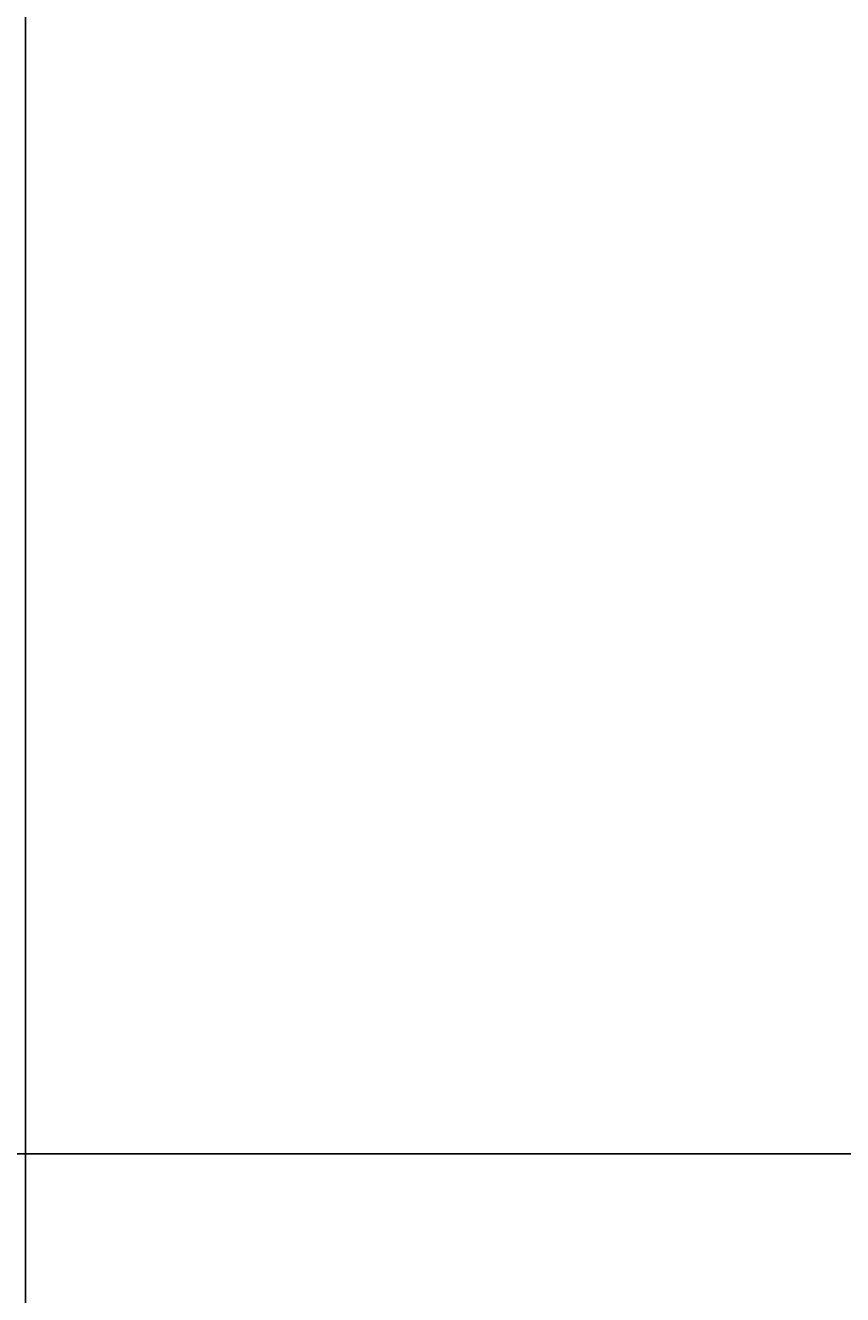
# Model space of a CAD drawing. Units: inches. Extents: x 37 to 824, y -700 to 234.
# Tile 52 of 77: x 170 to 204, y 107 to 160. Entities that reach past the tile are written whole.
import ezdxf

# ---------------------------------------------------------------- set-up
doc = ezdxf.new("R2010")
doc.units = ezdxf.units.IN
doc.header["$MEASUREMENT"] = 0
doc.layers.add('A-ANNO-DIMS', color=2, linetype='Continuous', lineweight=18)
doc.styles.get("Standard").update_dxf_attribs({"font": 'arial.ttf'})
doc.dimstyles.get("Standard").update_dxf_attribs({"dimtxt": 0.18, "dimasz": 0.18, "dimexe": 0.18, "dimexo": 0.0625, "dimgap": 0.09, "dimtad": 0, "dimtih": 1, "dimtoh": 1, "dimdec": 1, "dimzin": 0, "dimdsep": 46, "dimlunit": 4, "dimtxsty": 'Standard', "dimcen": 0.09, "dimadec": 0, "dimazin": 0, "dimtfac": 1, "dimtdec": 1, "dimtofl": 0, "dimtmove": 0, "dimatfit": 3, "dimfxl": 1, "dimtolj": 1, "dimtzin": 0, "dimarcsym": 0})

# ---------------------------------------------------------------- blocks, each defined once
blk = doc.blocks.new('*D60')
at = {"layer": 'A-ANNO-DIMS', "color": 0, "lineweight": -2, "ltscale": 0.5, "transparency": 16777216}
for p, q in [((419.015, 113.09), (78.159, 113.09)), ((78.339, 112.91), (78.339, 98.772)), ((78.339, 84.27), (78.339, 98.409)), ((419.015, 84.09), (78.159, 84.09))]:
    blk.add_line(p, q, dxfattribs=at)
at = {"layer": 'A-ANNO-DIMS', "color": 0, "ltscale": 0.5, "transparency": 16777216}
for points in [[(78.309, 112.91), (78.369, 112.91), (78.339, 113.09)], [(78.309, 84.27), (78.369, 84.27), (78.339, 84.09)]]:
    blk.add_solid(points, dxfattribs=at)
at = {"layer": 'Defpoints', "color": 0, "ltscale": 0.5, "transparency": 16777216}
for p in [(78.339, 113.09), (419.077, 113.09), (419.077, 84.09)]:
    blk.add_point(p, dxfattribs=at)
at = {"layer": 'A-ANNO-DIMS', "color": 0, "ltscale": 0.5, "transparency": 16777216, "insert": (78.339, 98.59), "char_height": 0.18, "attachment_point": 5}
blk.add_mtext('\\A1;2\'-5"', dxfattribs=at)
blk = doc.blocks.new('*D72')
at = {"layer": 'A-ANNO-DIMS', "color": 0, "lineweight": -2, "ltscale": 0.5, "transparency": 16777216}
for p, q in [((170.077, 84.153), (170.077, 234.17)), ((250.19, 84.153), (250.19, 234.17)), ((170.257, 233.99), (209.804, 233.99)), ((250.01, 233.99), (210.463, 233.99))]:
    blk.add_line(p, q, dxfattribs=at)
at = {"layer": 'A-ANNO-DIMS', "color": 0, "ltscale": 0.5, "transparency": 16777216}
for points in [[(170.257, 234.02), (170.257, 233.96), (170.077, 233.99)], [(250.01, 234.02), (250.01, 233.96), (250.19, 233.99)]]:
    blk.add_solid(points, dxfattribs=at)
at = {"layer": 'Defpoints', "color": 0, "ltscale": 0.5, "transparency": 16777216}
for p in [(250.19, 233.99), (170.077, 84.09), (250.19, 84.09)]:
    blk.add_point(p, dxfattribs=at)
at = {"layer": 'A-ANNO-DIMS', "color": 0, "ltscale": 0.5, "transparency": 16777216, "insert": (210.133, 233.99), "char_height": 0.18, "attachment_point": 5}
blk.add_mtext('\\A1;6\'-8"', dxfattribs=at)
blk = doc.blocks.new('*D84')
at = {"layer": 'A-ANNO-DIMS', "color": 0, "lineweight": -2, "ltscale": 0.5, "transparency": 16777216}
for p, q in [((170.077, -265.847), (170.077, 234.17)), ((210.077, -265.847), (210.077, 234.17)), ((170.257, 233.99), (189.748, 233.99)), ((209.897, 233.99), (190.406, 233.99))]:
    blk.add_line(p, q, dxfattribs=at)
at = {"layer": 'A-ANNO-DIMS', "color": 0, "ltscale": 0.5, "transparency": 16777216}
for points in [[(170.257, 234.02), (170.257, 233.96), (170.077, 233.99)], [(209.897, 234.02), (209.897, 233.96), (210.077, 233.99)]]:
    blk.add_solid(points, dxfattribs=at)
at = {"layer": 'Defpoints', "color": 0, "ltscale": 0.5, "transparency": 16777216}
for p in [(210.077, 233.99), (170.077, -265.91), (210.077, -265.91)]:
    blk.add_point(p, dxfattribs=at)
at = {"layer": 'A-ANNO-DIMS', "color": 0, "ltscale": 0.5, "transparency": 16777216, "insert": (190.077, 233.99), "char_height": 0.18, "attachment_point": 5}
blk.add_mtext('\\A1;3\'-4"', dxfattribs=at)
blk = doc.blocks.new('*D85')
at = {"layer": 'A-ANNO-DIMS', "color": 0, "lineweight": -2, "ltscale": 0.5, "transparency": 16777216}
for p, q in [((170.077, -356.847), (170.077, 234.17)), ((206.077, -356.847), (206.077, 234.17)), ((170.257, 233.99), (187.748, 233.99)), ((205.897, 233.99), (188.406, 233.99))]:
    blk.add_line(p, q, dxfattribs=at)
at = {"layer": 'A-ANNO-DIMS', "color": 0, "ltscale": 0.5, "transparency": 16777216}
for points in [[(170.257, 234.02), (170.257, 233.96), (170.077, 233.99)], [(205.897, 234.02), (205.897, 233.96), (206.077, 233.99)]]:
    blk.add_solid(points, dxfattribs=at)
at = {"layer": 'Defpoints', "color": 0, "ltscale": 0.5, "transparency": 16777216}
for p in [(206.077, 233.99), (170.077, -356.91), (206.077, -356.91)]:
    blk.add_point(p, dxfattribs=at)
at = {"layer": 'A-ANNO-DIMS', "color": 0, "ltscale": 0.5, "transparency": 16777216, "insert": (188.077, 233.99), "char_height": 0.18, "attachment_point": 5}
blk.add_mtext('\\A1;3\'-0"', dxfattribs=at)

msp = doc.modelspace()

# ---------------------------------------------------------------- dimensions: what is measured, and where the dimension line sits
at = {"layer": 'A-ANNO-DIMS', "ltscale": 0.5}
for base, p1, p2, picture, middle in [((250.19, 233.99), (170.077, 84.09), (250.19, 84.09), '*D72', (210.133, 233.99)), ((210.077, 233.99), (170.077, -265.91), (210.077, -265.91), '*D84', (190.077, 233.99)), ((206.077, 233.99), (170.077, -356.91), (206.077, -356.91), '*D85', (188.077, 233.99))]:
    dim = msp.add_linear_dim(base=base, p1=p1, p2=p2, dimstyle='Standard', override={"dimdec": 1, "dimlfac": 1, "dimrnd": 0, "dimzin": 1, "dimdsep": 46, "dimlunit": 4, "dimfrac": 2}, dxfattribs=at)
    dim.commit()
    dim.dimension.update_dxf_attribs({"geometry": picture, "text_midpoint": middle})
dim = msp.add_linear_dim(base=(78.339, 113.09), p1=(419.077, 84.09), p2=(419.077, 113.09), angle=90, dimstyle='Standard', override={"dimdec": 1, "dimlfac": 1, "dimrnd": 0, "dimzin": 1, "dimdsep": 46, "dimlunit": 4, "dimfrac": 2}, dxfattribs=at)
dim.commit()
dim.dimension.update_dxf_attribs({"geometry": '*D60', "text_midpoint": (78.339, 98.59)})

doc.saveas('drawing.dxf')
